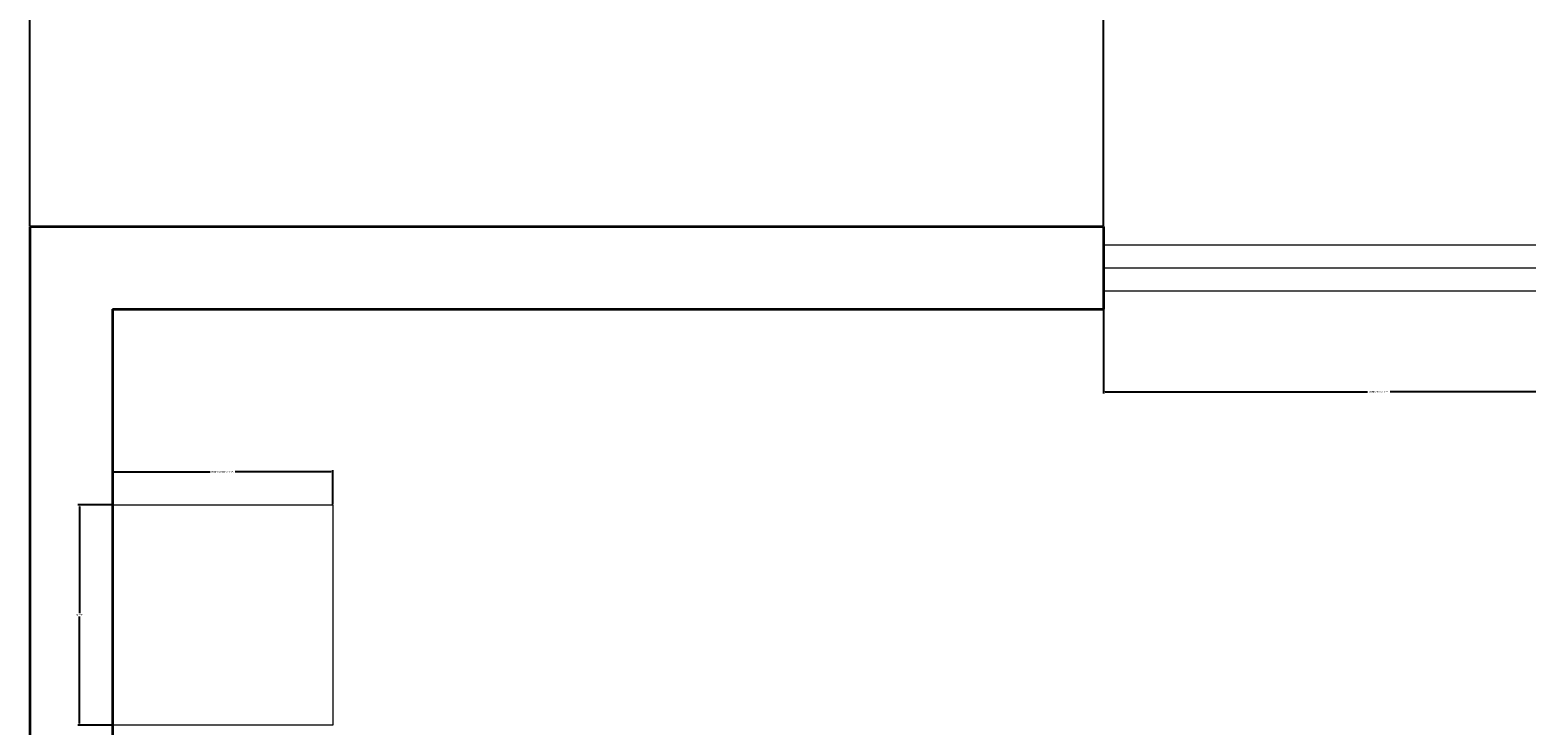
# Model space of a CAD drawing. Units: inches. Extents: x -4843 to -3402, y -164 to 3629.
# Tile 16 of 22: x -4596 to -4433, y 966 to 1042. Entities that reach past the tile are written whole.
import ezdxf

# ---------------------------------------------------------------- set-up
doc = ezdxf.new("R2010")
doc.units = ezdxf.units.IN
for name, color, linetype, lineweight in [('A-ANNO-DIMS', 2, 'Continuous', 18), ('furniture', 6, 'Continuous', 18), ('walls', 7, 'Continuous', 35), ('windows', 1, 'Continuous', 18)]:
    doc.layers.add(name, color=color, linetype=linetype, lineweight=lineweight)
doc.styles.get("Standard").update_dxf_attribs({"font": 'arial.ttf'})
doc.dimstyles.get("Standard").update_dxf_attribs({"dimtxt": 0.18, "dimasz": 0.18, "dimexe": 0.18, "dimexo": 0.0625, "dimgap": 0.09, "dimtad": 0, "dimtih": 1, "dimtoh": 1, "dimdec": 4, "dimzin": 0, "dimdsep": 46, "dimtxsty": 'Standard', "dimcen": 0.09, "dimadec": 0, "dimazin": 0, "dimtfac": 1, "dimtdec": 4, "dimtofl": 0, "dimtmove": 0, "dimatfit": 3, "dimfxl": 1, "dimtolj": 1, "dimtzin": 0, "dimarcsym": 0})

# ---------------------------------------------------------------- blocks, each defined once
blk = doc.blocks.new('window')
at = {"layer": 'windows'}
for p, q in [((0, 7), (60, 7)), ((0, 4.5), (60, 4.5)), ((0, 2), (60, 2))]:
    blk.add_line(p, q, dxfattribs=at)
for points in [[(0, 9), (0, 0)], [(60, 0), (60, 9)]]:
    blk.add_lwpolyline(points, dxfattribs=at)
blk = doc.blocks.new('NIGHTSTAND-24IN')
blk.add_lwpolyline([(0, 24), (24, 24), (24, 0), (0, 0)], close=True)
blk = doc.blocks.new('*D36')
at = {"layer": 'A-ANNO-DIMS', "color": 0, "lineweight": -2, "transparency": 16777216}
for p, q in [((-4478.78, 1011.29), (-4478.78, 1002.17)), ((-4418.78, 1011.29), (-4418.78, 1002.17)), ((-4478.6, 1002.35), (-4450.02, 1002.35)), ((-4418.96, 1002.35), (-4447.55, 1002.35))]:
    blk.add_line(p, q, dxfattribs=at)
at = {"layer": 'A-ANNO-DIMS', "color": 0, "transparency": 16777216}
for points in [[(-4478.6, 1002.38), (-4478.6, 1002.32), (-4478.78, 1002.35)], [(-4418.96, 1002.38), (-4418.96, 1002.32), (-4418.78, 1002.35)]]:
    blk.add_solid(points, dxfattribs=at)
at = {"layer": 'Defpoints', "color": 0, "transparency": 16777216}
for p in [(-4478.78, 1011.35), (-4418.78, 1011.35), (-4418.78, 1002.35)]:
    blk.add_point(p, dxfattribs=at)
at = {"layer": 'A-ANNO-DIMS', "color": 0, "transparency": 16777216, "insert": (-4448.78, 1002.35), "char_height": 0.18, "attachment_point": 5}
blk.add_mtext('\\A1;WINDOW A 60 TYP.', dxfattribs=at)
blk = doc.blocks.new('*D46')
at = {"layer": 'A-ANNO-DIMS', "color": 0, "lineweight": -2, "transparency": 16777216}
for p, q in [((-4586.78, 990.08), (-4586.78, 993.8)), ((-4586.6, 993.62), (-4576.16, 993.62)), ((-4562.96, 993.62), (-4573.41, 993.62)), ((-4562.78, 990.08), (-4562.78, 993.8))]:
    blk.add_line(p, q, dxfattribs=at)
at = {"layer": 'A-ANNO-DIMS', "color": 0, "transparency": 16777216}
for points in [[(-4586.6, 993.65), (-4586.6, 993.59), (-4586.78, 993.62)], [(-4562.96, 993.65), (-4562.96, 993.59), (-4562.78, 993.62)]]:
    blk.add_solid(points, dxfattribs=at)
at = {"layer": 'Defpoints', "color": 0, "transparency": 16777216}
for p in [(-4562.78, 993.62), (-4586.78, 990.02), (-4562.78, 990.02)]:
    blk.add_point(p, dxfattribs=at)
at = {"layer": 'A-ANNO-DIMS', "color": 0, "transparency": 16777216, "insert": (-4574.78, 993.62), "char_height": 0.18, "attachment_point": 5}
blk.add_mtext('\\A1;NIGHTSTAND 24 TYP.', dxfattribs=at)
blk = doc.blocks.new('*D47')
at = {"layer": 'A-ANNO-DIMS', "color": 0, "lineweight": -2, "transparency": 16777216}
for p, q in [((-4586.85, 990.02), (-4590.56, 990.02)), ((-4590.38, 989.84), (-4590.38, 978.2)), ((-4590.38, 966.2), (-4590.38, 977.84)), ((-4586.85, 966.02), (-4590.56, 966.02))]:
    blk.add_line(p, q, dxfattribs=at)
at = {"layer": 'A-ANNO-DIMS', "color": 0, "transparency": 16777216}
for points in [[(-4590.41, 989.84), (-4590.35, 989.84), (-4590.38, 990.02)], [(-4590.41, 966.2), (-4590.35, 966.2), (-4590.38, 966.02)]]:
    blk.add_solid(points, dxfattribs=at)
at = {"layer": 'Defpoints', "color": 0, "transparency": 16777216}
for p in [(-4590.38, 990.02), (-4586.78, 990.02), (-4586.78, 966.02)]:
    blk.add_point(p, dxfattribs=at)
at = {"layer": 'A-ANNO-DIMS', "color": 0, "transparency": 16777216, "insert": (-4590.38, 978.02), "char_height": 0.18, "attachment_point": 5}
blk.add_mtext('\\A1;24 TYP.', dxfattribs=at)
blk = doc.blocks.new('*D69')
at = {"layer": 'A-ANNO-DIMS', "color": 0, "lineweight": -2, "transparency": 16777216}
for p, q in [((-4595.78, 1020.42), (-4595.78, 1392.95)), ((-4595.6, 1392.77), (-4537.56, 1392.77)), ((-4478.96, 1392.77), (-4537, 1392.77)), ((-4478.78, 1020.42), (-4478.78, 1392.95))]:
    blk.add_line(p, q, dxfattribs=at)
at = {"layer": 'A-ANNO-DIMS', "color": 0, "transparency": 16777216}
for points in [[(-4595.6, 1392.8), (-4595.6, 1392.74), (-4595.78, 1392.77)], [(-4478.96, 1392.8), (-4478.96, 1392.74), (-4478.78, 1392.77)]]:
    blk.add_solid(points, dxfattribs=at)
at = {"layer": 'Defpoints', "color": 0, "transparency": 16777216}
for p in [(-4478.78, 1392.77), (-4595.78, 1020.35), (-4478.78, 1020.35)]:
    blk.add_point(p, dxfattribs=at)
at = {"layer": 'A-ANNO-DIMS', "color": 0, "transparency": 16777216, "insert": (-4537.28, 1392.77), "char_height": 0.18, "attachment_point": 5}
blk.add_mtext('\\A1;117', dxfattribs=at)

msp = doc.modelspace()

# ---------------------------------------------------------------- linework, layer by layer
at = {"layer": 'walls'}
for p, q in [((-4595.78, 1020.35), (-4595.78, 897.35)), ((-4595.78, 1020.35), (-4478.78, 1020.35)), ((-4586.78, 1011.35), (-4586.78, 897.35)), ((-4586.78, 1011.35), (-4478.78, 1011.35))]:
    msp.add_line(p, q, dxfattribs=at)
msp.add_lwpolyline([(-4478.78, 1020.35), (-4478.78, 1011.35)], dxfattribs=at)

# ---------------------------------------------------------------- block references
at = {"layer": 'furniture'}
msp.add_blockref('NIGHTSTAND-24IN', (-4586.78, 966.02), dxfattribs=at)
at = {"layer": 'windows'}
msp.add_blockref('window', (-4478.78, 1011.35), dxfattribs=at)

# ---------------------------------------------------------------- dimensions: what is measured, and where the dimension line sits
at = {"layer": 'A-ANNO-DIMS'}
dim = msp.add_linear_dim(base=(-4478.78, 1392.77), p1=(-4595.78, 1020.35), p2=(-4478.78, 1020.35), dimstyle='Standard', override={"dimdec": 0, "dimlfac": 1, "dimrnd": 0, "dimzin": 0, "dimdsep": 46, "dimlunit": 2}, dxfattribs=at)
dim.commit()
dim.dimension.update_dxf_attribs({"geometry": '*D69', "text_midpoint": (-4537.28, 1392.77)})
for base, p1, p2, text, picture, middle in [((-4418.78, 1002.35), (-4478.78, 1011.35), (-4418.78, 1011.35), 'WINDOW A <> TYP.', '*D36', (-4448.78, 1002.35)), ((-4562.78, 993.62), (-4586.78, 990.02), (-4562.78, 990.02), 'NIGHTSTAND <> TYP.', '*D46', (-4574.78, 993.62))]:
    dim = msp.add_linear_dim(base=base, p1=p1, p2=p2, text=text, dimstyle='Standard', override={"dimdec": 0, "dimlfac": 1, "dimrnd": 0, "dimzin": 0, "dimdsep": 46, "dimlunit": 2}, dxfattribs=at)
    dim.commit()
    dim.dimension.update_dxf_attribs({"geometry": picture, "text_midpoint": middle})
dim = msp.add_linear_dim(base=(-4590.38, 990.02), p1=(-4586.78, 966.02), p2=(-4586.78, 990.02), angle=90, text='<> TYP.', dimstyle='Standard', override={"dimdec": 0, "dimlfac": 1, "dimrnd": 0, "dimzin": 0, "dimdsep": 46, "dimlunit": 2}, dxfattribs=at)
dim.commit()
dim.dimension.update_dxf_attribs({"geometry": '*D47', "text_midpoint": (-4590.38, 978.02)})

doc.saveas('drawing.dxf')
